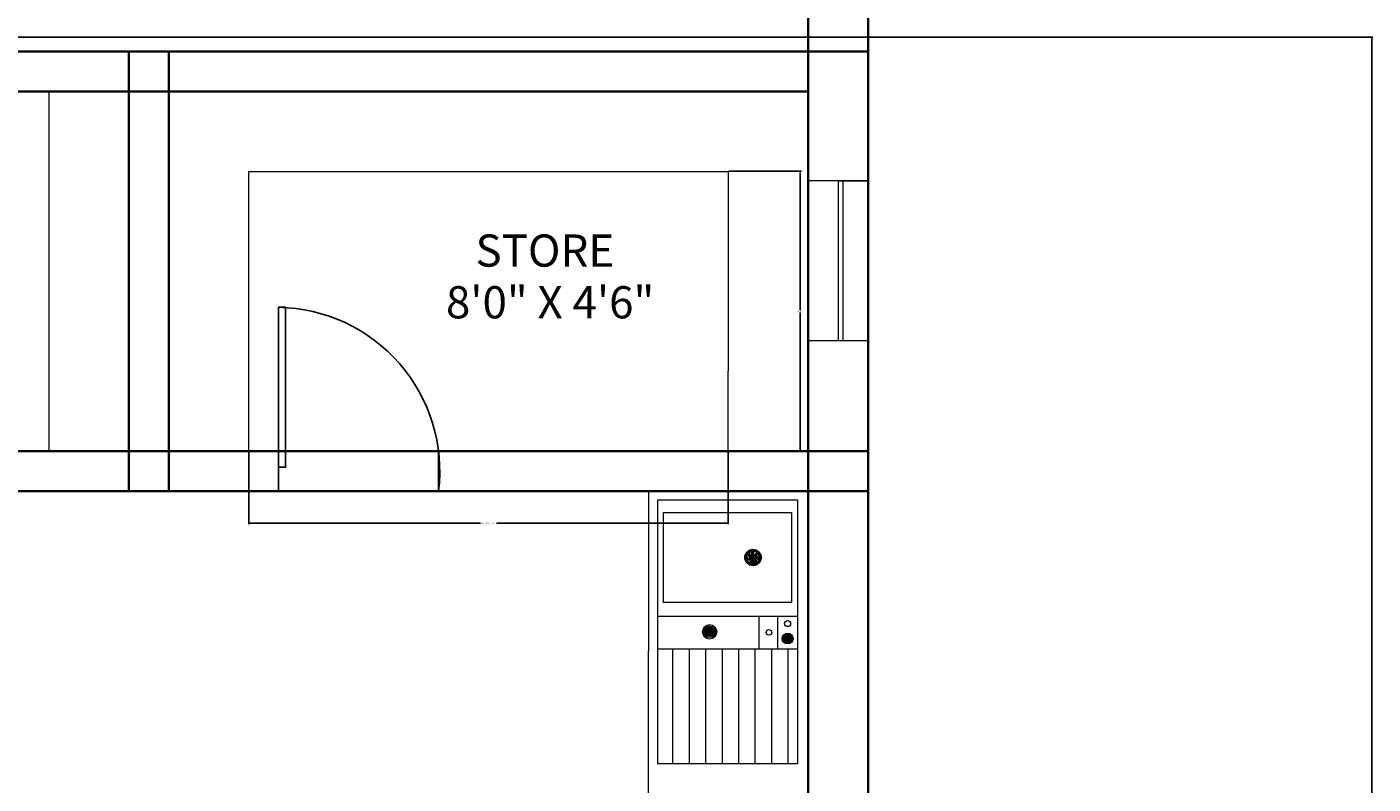
# Model space of a CAD drawing. Units: inches. Extents: x -61 to 1599, y -1316 to 257.
# Tile 197 of 204: x 1396 to 1599, y -279 to -166. Entities that reach past the tile are written whole.
import ezdxf

# ---------------------------------------------------------------- set-up
doc = ezdxf.new("R2010")
doc.units = ezdxf.units.IN
doc.header["$MEASUREMENT"] = 0
doc.linetypes.add('ACAD_ISO02W100', pattern=[15, 12, -3])
for name, color, linetype, lineweight in [('A-ANNO-DIMS', 2, 'Continuous', 18), ('A-AREA-IDEN', 1, 'Continuous', 18), ('A-FLOR-CASE', 8, 'Continuous', 18), ('A-FLOR-FIXT', 8, 'Continuous', 18), ('A-WALL-JAMB', 4, 'ACAD_ISO02W100', 25), ('DOORS', 2, 'Continuous', 25), ('WALLS', 4, 'Continuous', 35), ('WINDOWS', 220, 'Continuous', 18)]:
    doc.layers.add(name, color=color, linetype=linetype, lineweight=lineweight)
doc.layers.add('FUR', color=83, linetype='Continuous')
doc.styles.get("Standard").update_dxf_attribs({"font": 'arial.ttf'})
doc.dimstyles.get("Standard").update_dxf_attribs({"dimtxt": 0.18, "dimasz": 0.18, "dimexe": 0.18, "dimexo": 0.0625, "dimgap": 0.09, "dimtad": 0, "dimtih": 1, "dimtoh": 1, "dimdec": 0, "dimzin": 0, "dimdsep": 46, "dimlunit": 3, "dimtxsty": 'Standard', "dimcen": 0.09, "dimadec": 0, "dimazin": 0, "dimtfac": 1, "dimtdec": 0, "dimtofl": 0, "dimtmove": 0, "dimatfit": 3, "dimfxl": 1, "dimtolj": 1, "dimtzin": 0, "dimarcsym": 0})

# ---------------------------------------------------------------- blocks, each defined once
blk = doc.blocks.new('DOOR-SWING-24')
blk.add_line((0, 0), (0, 3.6))
blk.add_lwpolyline([(0, 0), (0, -24), (1.05, -24), (1.05, 0)], close=True)
blk.add_arc((-0.44, 0.62), 24.62, 271.0259, 6.9559)
blk = doc.blocks.new('WIN-24IN')
for p, q in [((0, 4.5), (0, 9)), ((0, 9), (0, 0)), ((24, 9), (24, 0)), ((0, 5.19), (24, 5.19)), ((0, 4.5), (24, 4.5))]:
    blk.add_line(p, q)
blk = doc.blocks.new('*U268')
at = {"layer": 'FUR'}
blk.add_line((0.41, 1.36), (0.41, 0.68), dxfattribs=at)
blk.add_open_spline([(0.41, 1.36), (0.24, 1.25), (-0.09, 1.02), (0.41, 0.7), (0.83, 0.34), (0.55, 0.11), (0.41, 0)], degree=3, knots=[0, 0, 0, 0, 0.474547, 0.949094, 1.393355, 1.837616, 1.837616, 1.837616, 1.837616], dxfattribs=at)
blk = doc.blocks.new('*U269')
at = {"layer": 'FUR', "transparency": 16777216}
for p, rotation in [((531.82, -257.55), 308.5714285714286), ((532.89, -258.18), 51.42857142857144), ((532.03, -256.89), 257.1428571428571), ((533.36, -257.68), 102.8571428571428), ((532.68, -256.65), 205.7142857142857), ((533.27, -257), 154.2857142857143)]:
    blk.add_blockref('*U268', p, dxfattribs=dict(at, rotation=rotation))
blk.add_blockref('*U268', (532.2, -258.12), dxfattribs=at)
blk = doc.blocks.new('*U270')
at = {"layer": 'FUR'}
blk.add_line((0.74, 2.46), (0.74, 1.23), dxfattribs=at)
blk.add_open_spline([(0.74, 2.46), (0.44, 2.26), (-0.16, 1.84), (0.74, 1.26), (1.5, 0.61), (0.99, 0.2), (0.74, 0)], degree=3, knots=[0, 0, 0, 0, 0.85637, 1.712739, 2.514455, 3.316171, 3.316171, 3.316171, 3.316171], dxfattribs=at)
blk = doc.blocks.new('*U271')
at = {"layer": 'FUR', "transparency": 16777216}
for p, rotation in [((959.72, -464.77), 308.5714285714286), ((961.65, -465.92), 51.42857142857144), ((960.11, -463.59), 257.1428571428571), ((962.51, -465.02), 102.8571428571428), ((961.27, -463.15), 205.7142857142858), ((962.34, -463.79), 154.2857142857143)]:
    blk.add_blockref('*U270', p, dxfattribs=dict(at, rotation=rotation))
blk.add_blockref('*U270', (960.41, -465.81), dxfattribs=at)
blk = doc.blocks.new('*U266')
at = {"layer": 'FUR'}
blk.add_line((0.41, 1.36), (0.41, 0.68), dxfattribs=at)
blk.add_open_spline([(0.41, 1.36), (0.24, 1.25), (-0.09, 1.02), (0.41, 0.7), (0.83, 0.34), (0.55, 0.11), (0.41, 0)], degree=3, knots=[0, 0, 0, 0, 0.474547, 0.949094, 1.393355, 1.837616, 1.837616, 1.837616, 1.837616], dxfattribs=at)
blk = doc.blocks.new('*U267')
at = {"layer": 'FUR', "transparency": 16777216}
for p, rotation in [((531.82, -257.55), 308.5714285714286), ((532.89, -258.18), 51.42857142857144), ((532.03, -256.89), 257.1428571428571), ((533.36, -257.68), 102.8571428571428), ((532.68, -256.65), 205.7142857142857), ((533.27, -257), 154.2857142857143)]:
    blk.add_blockref('*U266', p, dxfattribs=dict(at, rotation=rotation))
blk.add_blockref('*U266', (532.2, -258.12), dxfattribs=at)
blk = doc.blocks.new('SINK-WITH-DRAINBOARD')
for p, q in [((14.29, 30.97), (14.29, 29.74)), ((0, 22.17), (20.98, 22.17)), ((15.24, 17.27), (15.24, 22.17)), ((17.97, 22.17), (17.97, 17.27)), ((7.79, 19.82), (7.79, 19.14)), ((19.48, 18.8), (19.48, 18.12)), ((0, 17.27), (20.98, 17.27)), ((2.27, 0), (2.27, 17.27)), ((4.74, 0), (4.74, 17.27)), ((7.21, 0), (7.21, 17.27)), ((9.69, 0), (9.69, 17.27)), ((12.16, 0), (12.16, 17.27)), ((14.63, 0), (14.63, 17.27)), ((17.1, 0), (17.1, 17.27)), ((19.58, 0), (19.58, 17.27))]:
    blk.add_line(p, q)
for points in [[(20.98, 0), (0, 0), (0, 39.63), (20.98, 39.63)], [(20.07, 24.22), (0.86, 24.22), (0.86, 37.7), (20.07, 37.7)]]:
    blk.add_lwpolyline(points, close=True)
for centre, radius in [((14.29, 30.97), 1.23), ((7.78, 19.81), 1.08), ((7.78, 19.81), 0.877), ((7.79, 19.82), 0.682), ((19.48, 21.05), 0.455), ((16.69, 19.72), 0.419), ((19.48, 18.8), 0.816), ((19.48, 18.8), 0.816), ((19.48, 18.8), 0.682)]:
    blk.add_circle(centre, radius)
for name, p in [('*U271', (-946.85, 495.54)), ('*U269', (-524.82, 277.26)), ('*U267', (-513.12, 276.24))]:
    blk.add_blockref(name, p)
blk = doc.blocks.new('STORE-SHELVING')
for p, q in [((0, 42), (72, 42)), ((0, 12), (0, 42)), ((72, 42), (72, 12)), ((0, 0), (0, 12)), ((72, 0), (72, 12))]:
    blk.add_line(p, q)
blk = doc.blocks.new('*D674')
at = {"layer": 'A-ANNO-DIMS', "color": 0, "lineweight": -2, "transparency": 16777216}
for p, q in [((1429.7, -229.39), (1429.7, -240.3)), ((1501.7, -229.39), (1501.7, -240.3)), ((1429.88, -240.12), (1464.5, -240.12)), ((1501.52, -240.12), (1466.9, -240.12))]:
    blk.add_line(p, q, dxfattribs=at)
at = {"layer": 'A-ANNO-DIMS', "color": 0, "transparency": 16777216}
for points in [[(1429.88, -240.09), (1429.88, -240.15), (1429.7, -240.12)], [(1501.52, -240.09), (1501.52, -240.15), (1501.7, -240.12)]]:
    blk.add_solid(points, dxfattribs=at)
at = {"layer": 'DEFPOINTS', "color": 0, "transparency": 16777216}
for p in [(1429.7, -229.32), (1501.7, -229.32), (1501.7, -240.12)]:
    blk.add_point(p, dxfattribs=at)
at = {"layer": 'A-ANNO-DIMS', "color": 0, "transparency": 16777216, "insert": (1465.7, -240.12), "char_height": 0.18, "attachment_point": 5}
blk.add_mtext('\\A1;SHELVING 72 TYP.', dxfattribs=at)
blk = doc.blocks.new('*D675')
at = {"layer": 'A-ANNO-DIMS', "color": 0, "lineweight": -2, "transparency": 16777216}
for p, q in [((1501.77, -187.32), (1512.68, -187.32)), ((1512.5, -187.5), (1512.5, -208.14)), ((1512.5, -229.14), (1512.5, -208.5)), ((1501.77, -229.32), (1512.68, -229.32))]:
    blk.add_line(p, q, dxfattribs=at)
at = {"layer": 'A-ANNO-DIMS', "color": 0, "transparency": 16777216}
for points in [[(1512.47, -187.5), (1512.53, -187.5), (1512.5, -187.32)], [(1512.47, -229.14), (1512.53, -229.14), (1512.5, -229.32)]]:
    blk.add_solid(points, dxfattribs=at)
at = {"layer": 'DEFPOINTS', "color": 0, "transparency": 16777216}
for p in [(1501.7, -187.32), (1512.5, -187.32), (1501.7, -229.32)]:
    blk.add_point(p, dxfattribs=at)
at = {"layer": 'A-ANNO-DIMS', "color": 0, "transparency": 16777216, "insert": (1512.5, -208.32), "char_height": 0.18, "attachment_point": 5}
blk.add_mtext('\\A1;42 TYP.', dxfattribs=at)
blk = doc.blocks.new('*D698')
at = {"layer": 'A-ANNO-DIMS', "color": 0, "lineweight": -2, "transparency": 16777216}
for p, q in [((644.77, -167.17), (1598.48, -167.17)), ((1598.3, -167.35), (1598.3, -363.99)), ((1598.3, -560.99), (1598.3, -364.35)), ((644.77, -561.17), (1598.48, -561.17))]:
    blk.add_line(p, q, dxfattribs=at)
at = {"layer": 'A-ANNO-DIMS', "color": 0, "transparency": 16777216}
for points in [[(1598.27, -167.35), (1598.33, -167.35), (1598.3, -167.17)], [(1598.27, -560.99), (1598.33, -560.99), (1598.3, -561.17)]]:
    blk.add_solid(points, dxfattribs=at)
at = {"layer": 'DEFPOINTS', "color": 0, "transparency": 16777216}
for p in [(644.7, -167.17), (1598.3, -167.17), (644.7, -561.17)]:
    blk.add_point(p, dxfattribs=at)
at = {"layer": 'A-ANNO-DIMS', "color": 0, "transparency": 16777216, "insert": (1598.3, -364.17), "char_height": 0.18, "attachment_point": 5}
blk.add_mtext('\\A1;394', dxfattribs=at)

msp = doc.modelspace()

# ---------------------------------------------------------------- linework, layer by layer
at = {"layer": 'A-FLOR-CASE'}
for p in [(1489.7028, -235.3229), (1489.7028, -348.3229)]:
    msp.add_line(p, (1489.7028, -259.3229), dxfattribs=at)
msp.add_lwpolyline([(1411.7028, -229.3229), (1399.7505, -229.3229), (1399.7505, -175.3229), (1411.7028, -175.3229)], close=True, dxfattribs=at)
at = {"layer": 'A-WALL-JAMB'}
for p, q in [((1434.2028, -235.3229), (1434.2028, -229.3229)), ((1458.2028, -235.3229), (1458.1983, -229.3229))]:
    msp.add_line(p, q, dxfattribs=at)
at = {"layer": 'WALLS'}
for p, q in [((1513.7028, -13.3229), (1513.7028, -175.3229)), ((1522.7028, -441.3229), (1522.7028, -67.169)), ((1375.7028, -169.3229), (1522.7028, -169.3229)), ((1411.7028, -235.3229), (1411.7028, -169.3229)), ((1417.7028, -235.3229), (1417.7028, -169.3229)), ((1351.7028, -175.3229), (1411.7028, -175.3229)), ((1411.7028, -175.3229), (1417.7028, -175.3229)), ((1417.7028, -175.3229), (1513.7028, -175.3229)), ((1513.7028, -282.3229), (1513.7028, -175.3229)), ((1345.7028, -229.3229), (1522.7028, -229.3229)), ((1411.7028, -229.3229), (1522.7028, -229.3229)), ((1345.7028, -235.3229), (1522.7028, -235.3229)), ((1411.7028, -235.3229), (1522.7028, -235.3229))]:
    msp.add_line(p, q, dxfattribs=at)

# ---------------------------------------------------------------- block references
at = {"layer": 'A-FLOR-CASE'}
msp.add_blockref('STORE-SHELVING', (1429.703, -229.323), dxfattribs=at)
at = {"layer": 'A-FLOR-FIXT'}
msp.add_blockref('SINK-WITH-DRAINBOARD', (1491.125, -276.244), dxfattribs=at)
at = {"layer": 'DOORS', "extrusion": (0, 0, -1), "zscale": -1, "rotation": 180}
msp.add_blockref('DOOR-SWING-24', (-1434.2028, -231.7229), dxfattribs=at)
at = {"layer": 'WINDOWS', "rotation": 270.0000000000002}
msp.add_blockref('WIN-24IN', (1513.7027, -188.7656), dxfattribs=at)

# ---------------------------------------------------------------- texts
at = {"layer": 'A-AREA-IDEN'}
for s, height, p in [('   STORE', 4.8321, (1459.3179, -201.6263)), ('8\'0" X 4\'6"', 4.832098, (1459.3179, -209.3886))]:
    msp.add_text(s, height=height, dxfattribs=at).set_placement(p)

# ---------------------------------------------------------------- dimensions: what is measured, and where the dimension line sits
at = {"layer": 'A-ANNO-DIMS'}
dim = msp.add_linear_dim(base=(1598.3028, -167.169), p1=(644.7028, -561.169), p2=(644.7028, -167.169), angle=90, dimstyle='Standard', override={"dimdec": 0, "dimlfac": 1, "dimrnd": 0, "dimzin": 0, "dimdsep": 46, "dimlunit": 2}, dxfattribs=at)
dim.commit()
dim.dimension.update_dxf_attribs({"geometry": '*D698', "text_midpoint": (1598.3028, -364.169)})
dim = msp.add_linear_dim(base=(1512.5028, -187.3229), p1=(1501.7028, -229.3229), p2=(1501.7028, -187.3229), angle=90, text='<> TYP.', dimstyle='Standard', override={"dimdec": 0, "dimlfac": 1, "dimrnd": 0, "dimzin": 0, "dimdsep": 46, "dimlunit": 2}, dxfattribs=at)
dim.commit()
dim.dimension.update_dxf_attribs({"geometry": '*D675', "text_midpoint": (1512.5028, -208.3229)})
dim = msp.add_linear_dim(base=(1501.7028, -240.1229), p1=(1429.7028, -229.3229), p2=(1501.7028, -229.3229), text='SHELVING <> TYP.', dimstyle='Standard', override={"dimdec": 0, "dimlfac": 1, "dimrnd": 0, "dimzin": 0, "dimdsep": 46, "dimlunit": 2}, dxfattribs=at)
dim.commit()
dim.dimension.update_dxf_attribs({"geometry": '*D674', "text_midpoint": (1465.7028, -240.1229)})

doc.saveas('drawing.dxf')
